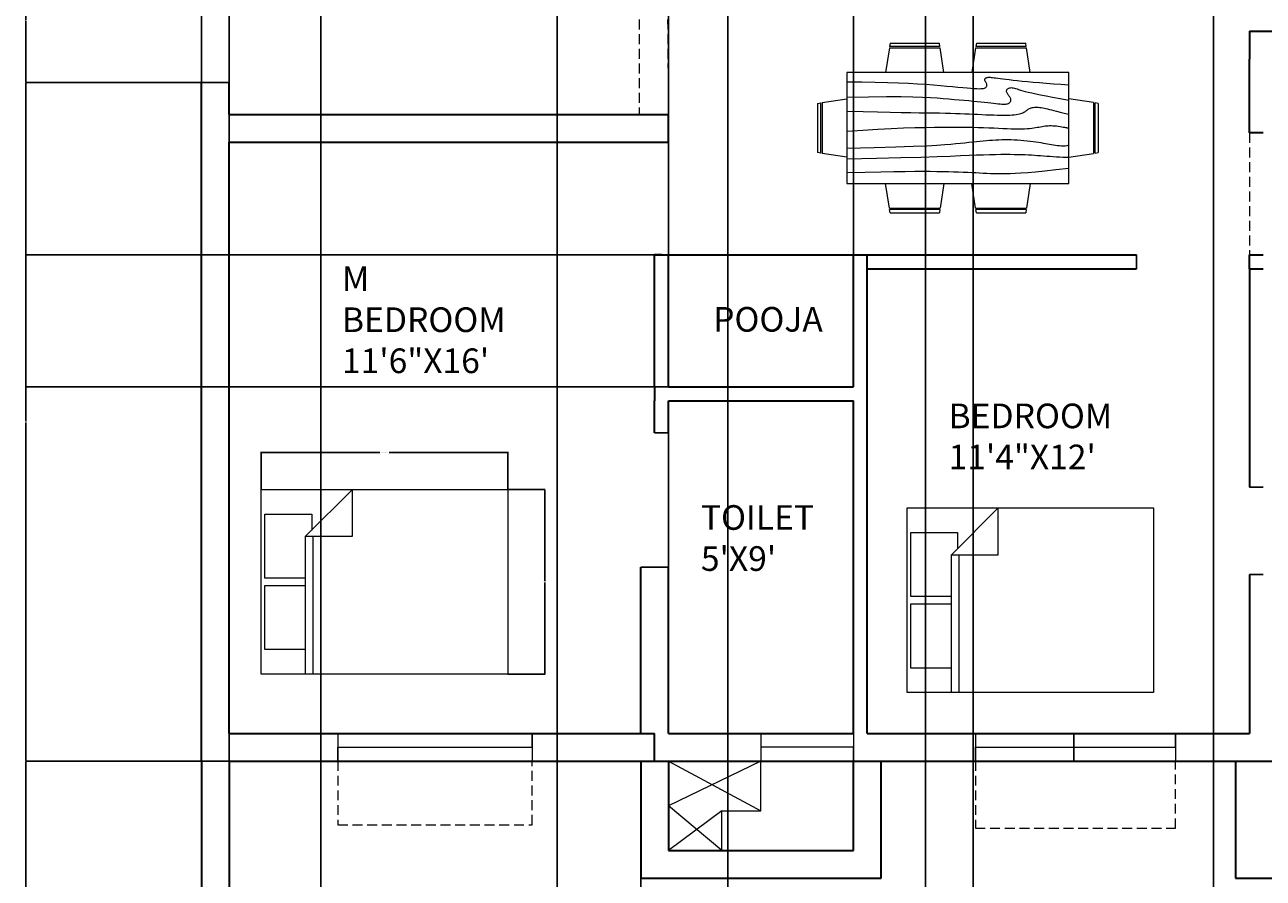
# Model space of a CAD drawing. Units: inches. Extents: x 276 to 912, y -567 to 621.
# Tile 5 of 7: x 276 to 678, y 65 to 342. Entities that reach past the tile are written whole.
import ezdxf

# ---------------------------------------------------------------- set-up
doc = ezdxf.new("R2010")
doc.units = ezdxf.units.IN
doc.linetypes.add('HIDDEN2', pattern=[4.7625, 3.175, -1.5875])
for name, color, linetype, lineweight in [('A-ANNO-DIMS', 2, 'Continuous', 18), ('A-AREA-IDEN', 7, 'Continuous', 18), ('A-DOOR', 3, 'Continuous', 25), ('A-FLOR-OVHD', 8, 'HIDDEN2', 13), ('A-FLOR-SHFT', 8, 'Continuous', 18), ('A-FURN', 8, 'Continuous', 18), ('A-GLAZ', 4, 'Continuous', 18), ('A-WALL', 7, 'Continuous', 35), ('A-WALL-HIDN', 8, 'HIDDEN2', 18)]:
    doc.layers.add(name, color=color, linetype=linetype, lineweight=lineweight)
doc.dimstyles.get("Standard").update_dxf_attribs({"dimtxt": 0.18, "dimasz": 0.18, "dimexe": 0.18, "dimexo": 0.0625, "dimgap": 0.09, "dimtad": 0, "dimtih": 1, "dimtoh": 1, "dimdec": 4, "dimzin": 0, "dimdsep": 46, "dimtxsty": 'Standard', "dimcen": 0.09, "dimadec": 0, "dimazin": 0, "dimtfac": 1, "dimtdec": 4, "dimtofl": 0, "dimtmove": 0, "dimatfit": 3, "dimfxl": 1, "dimtolj": 1, "dimtzin": 0, "dimarcsym": 0})

# ---------------------------------------------------------------- blocks, each defined once
blk = doc.blocks.new('Bed - Queen')
for p, q in [((0, -80.00003), (0, 0)), ((0, 0), (59.99999, 0)), ((59.99999, 0), (59.99999, -80.00003)), ((7.99999, -1.2), (28.79998, -1.2)), ((7.99999, -14.4), (7.99999, -1.2)), ((28.79998, -1.2), (28.79998, -14.4)), ((31.19999, -1.2), (51.99999, -1.2)), ((31.19999, -14.4), (31.19999, -1.2)), ((51.99999, -1.2), (51.99999, -16.4)), ((0, -14.4), (44.8, -14.4)), ((59.99999, -29.6), (44.8, -14.4)), ((44.8, -14.4), (44.8, -29.6)), ((44.8, -16.8), (0, -16.8)), ((51.99999, -16.4), (46.79936, -16.4)), ((44.8, -29.6), (59.99999, -29.6)), ((59.99999, -80.00003), (0, -80.00003))]:
    blk.add_line(p, q)
blk = doc.blocks.new('Dining Set - 36 x 72 in.')
for p, q in [((-22.2343, 26.00059), (-23.4847, 17.99762)), ((-22.2304, 26), (-5.7608, 26)), ((-22, 27.5), (-22.1562, 26.50042)), ((-5.8416, 26.5), (-22.1534, 26.5)), ((-22, 27.5), (-6, 27.5)), ((-5.8437, 26.49966), (-6, 27.5)), ((-4.5152, 17.99762), (-5.7655, 25.99926)), ((5.7657, 26.00059), (4.5153, 17.99762)), ((5.7696, 26), (22.2392, 26)), ((6, 27.5), (5.8438, 26.50042)), ((22.1584, 26.5), (5.8466, 26.5)), ((6, 27.5), (22, 27.5)), ((22.1563, 26.49966), (22, 27.5)), ((23.4848, 17.99762), (22.2345, 25.99926)), ((36, 18), (-36, 18)), ((-36, 18), (-36, -18)), ((36, -18), (36, 18)), ((-45.5, 8), (-44.5004, 8.15617)), ((-44.5, -8.15843), (-44.5, 8.15338)), ((-44.0006, 8.23428), (-35.9976, 9.48474)), ((-44, 8.23041), (-44, -8.23915)), ((44.0006, 8.23428), (35.9976, 9.48474)), ((44, 8.23041), (44, -8.23915)), ((44.5, -8.15843), (44.5, 8.15338)), ((45.5, 8), (44.5005, 8.15617)), ((-45.5, 8), (-45.5, -8)), ((45.5, 8), (45.5, -8)), ((-44.4997, -8.15631), (-45.5, -8)), ((44.4997, -8.15631), (45.5, -8)), ((-35.9976, -9.48476), (-43.9993, -8.2345)), ((35.9976, -9.48476), (43.9993, -8.2345)), ((-36, -18), (36, -18)), ((-22.2343, -26.0006), (-23.4847, -17.99762)), ((-4.5152, -17.99762), (-5.7655, -25.99928)), ((5.7657, -26.0006), (4.5153, -17.99762)), ((23.4848, -17.99762), (22.2345, -25.99928)), ((-22.2304, -26), (-5.7608, -26)), ((-22, -27.5), (-22.1562, -26.50044)), ((-5.8416, -26.5), (-22.1534, -26.5)), ((-22, -27.5), (-6, -27.5)), ((-5.8437, -26.49967), (-6, -27.5)), ((5.7696, -26), (22.2392, -26)), ((6, -27.5), (5.8438, -26.50044)), ((22.1584, -26.5), (5.8466, -26.5)), ((6, -27.5), (22, -27.5)), ((22.1563, -26.49967), (22, -27.5))]:
    blk.add_line(p, q)
for points in [[(-36, 15), (-31.1772, 14.97754), (-26.8079, 14.91406), (-22.8538, 14.81543), (-19.276, 14.6875), (-16.0362, 14.53613), (-13.0957, 14.36718), (-10.4159, 14.18652), (-7.9583, 14), (-5.6904, 13.81315), (-3.6035, 13.63021), (-1.6954, 13.45508), (0.0365, 13.29166), (1.5945, 13.14388), (2.9811, 13.01562), (4.1988, 12.9108), (5.25, 12.83333), (6.1393, 12.78613), (6.8802, 12.76823), (7.4883, 12.77767), (7.9792, 12.8125), (8.3685, 12.87077), (8.6719, 12.95052), (8.9049, 13.0498), (9.0833, 13.16666), (9.2205, 13.29899), (9.3216, 13.44401), (9.3895, 13.59879), (9.4271, 13.76041), (9.4373, 13.92594), (9.4232, 14.09245), (9.3875, 14.257), (9.3333, 14.41666), (9.2638, 14.56917), (9.1836, 14.71484), (9.0975, 14.85465), (9.0104, 14.98958), (8.9272, 15.1206), (8.8529, 15.2487), (8.7922, 15.37483), (8.75, 15.5), (8.7305, 15.62467), (8.7344, 15.74739), (8.7617, 15.86621), (8.8125, 15.97916), (8.8867, 16.08431), (8.9844, 16.17968), (9.1055, 16.26334), (9.25, 16.33333), (9.4189, 16.38802), (9.6172, 16.42708), (9.8506, 16.45052), (10.125, 16.45833), (10.4463, 16.45052), (10.8203, 16.42708), (11.2529, 16.38802), (11.75, 16.33333), (12.3184, 16.26318), (12.9694, 16.17838), (13.7151, 16.07991), (14.5677, 15.96875), (15.5395, 15.84586), (16.6426, 15.71224), (17.8893, 15.56884), (19.2917, 15.41666), (20.859, 15.25667), (22.5879, 15.08984), (24.4721, 14.91715), (26.5052, 14.73958), (28.6809, 14.5581), (30.9929, 14.3737), (33.4347, 14.18733), (36, 14)], [(-36, 10), (-28.9766, 10.14274), (-23.1725, 10.20442), (-18.4241, 10.19775), (-14.5677, 10.13541), (-11.4399, 10.03011), (-8.877, 9.89453), (-6.7154, 9.74137), (-4.7917, 9.58333), (-2.9698, 9.43082), (-1.2246, 9.28515), (0.4415, 9.14534), (2.026, 9.01041), (3.5266, 8.87939), (4.9408, 8.7513), (6.266, 8.62516), (7.5, 8.5), (8.6411, 8.37549), (9.6914, 8.2539), (10.6538, 8.13818), (11.5312, 8.03125), (12.3267, 7.93603), (13.043, 7.85547), (13.6831, 7.79248), (14.25, 7.75), (14.7471, 7.7303), (15.1797, 7.73307), (15.5537, 7.75732), (15.875, 7.80208), (16.1494, 7.86637), (16.3828, 7.94922), (16.5811, 8.04964), (16.75, 8.16666), (16.8944, 8.29915), (17.0143, 8.44531), (17.1089, 8.60319), (17.1771, 8.77083), (17.218, 8.94629), (17.2305, 9.1276), (17.2137, 9.31282), (17.1667, 9.5), (17.0895, 9.6875), (16.987, 9.875), (16.8649, 10.0625), (16.7292, 10.25), (16.5856, 10.4375), (16.4401, 10.625), (16.2985, 10.8125), (16.1667, 11), (16.05, 11.18733), (15.9518, 11.3737), (15.8752, 11.5581), (15.8229, 11.73958), (15.798, 11.91715), (15.8034, 12.08984), (15.842, 12.25667), (15.9167, 12.41666), (16.0295, 12.56836), (16.1784, 12.70833), (16.3605, 12.83268), (16.5729, 12.9375), (16.8127, 13.01888), (17.0768, 13.07291), (17.3625, 13.0957), (17.6667, 13.08333), (17.9894, 13.03312), (18.3418, 12.94726), (18.7382, 12.82918), (19.1927, 12.68229), (19.7195, 12.51001), (20.3327, 12.31575), (21.0465, 12.10294), (21.875, 11.875), (22.8357, 11.63354), (23.959, 11.37304), (25.2786, 11.08618), (26.8282, 10.76562), (28.6414, 10.40405), (30.752, 9.99414), (33.1936, 9.52856), (36, 9)], [(-36, 5.5), (-30.7157, 5.3348), (-26.069, 5.20963), (-21.9946, 5.11767), (-18.4271, 5.05208), (-15.3009, 5.00602), (-12.5508, 4.97265), (-10.1112, 4.94515), (-7.9167, 4.91666), (-5.909, 4.88167), (-4.0586, 4.83984), (-2.3429, 4.79215), (-0.7396, 4.73958), (0.7739, 4.6831), (2.22, 4.6237), (3.6213, 4.56233), (5, 4.5), (6.373, 4.43782), (7.7344, 4.3776), (9.0723, 4.32129), (10.375, 4.27083), (11.6309, 4.22819), (12.8281, 4.19531), (13.9551, 4.17415), (15, 4.16666), (15.954, 4.17448), (16.819, 4.19791), (17.6001, 4.23698), (18.3021, 4.29166), (18.9299, 4.36198), (19.4883, 4.44791), (19.9823, 4.54948), (20.4167, 4.66666), (20.7969, 4.79899), (21.1302, 4.94401), (21.4245, 5.09879), (21.6875, 5.26041), (21.9271, 5.42594), (22.1511, 5.59245), (22.3672, 5.757), (22.5834, 5.91666), (22.8065, 6.06868), (23.0404, 6.21093), (23.2879, 6.34147), (23.5521, 6.45833), (23.8358, 6.55957), (24.142, 6.64323), (24.4735, 6.70735), (24.8334, 6.75), (25.2235, 6.76969), (25.642, 6.76692), (26.0858, 6.74267), (26.5521, 6.69791), (27.0379, 6.63362), (27.5404, 6.55078), (28.0565, 6.45036), (28.5834, 6.33333), (29.1242, 6.19987), (29.7071, 6.04687), (30.3661, 5.87044), (31.1354, 5.66666), (32.0493, 5.43164), (33.142, 5.16146), (34.4475, 4.85221), (36, 4.5)], [(-36, -1), (-30.7915, -0.6591), (-26.0195, -0.38216), (-21.6519, -0.16284), (-17.6563, 0.00521), (-14.0005, 0.12833), (-10.6523, 0.21289), (-7.5796, 0.26522), (-4.75, 0.29166), (-2.134, 0.29793), (0.2878, 0.28711), (2.5317, 0.26163), (4.6146, 0.22396), (6.5529, 0.17651), (8.3633, 0.12174), (10.0623, 0.06209), (11.6667, 0), (13.1899, -0.06201), (14.6341, -0.1211), (15.9982, -0.17432), (17.2813, -0.21875), (18.4823, -0.25147), (19.6003, -0.26953), (20.6343, -0.27002), (21.5834, -0.25), (22.4481, -0.20768), (23.2357, -0.14584), (23.9549, -0.06836), (24.6146, 0.02083), (25.2235, 0.11784), (25.7904, 0.21875), (26.3241, 0.31966), (26.8334, 0.41666), (27.3265, 0.50618), (27.8099, 0.58593), (28.2894, 0.65397), (28.7709, 0.70833), (29.2601, 0.74707), (29.763, 0.76823), (30.2855, 0.76985), (30.8334, 0.75), (31.4088, 0.70784), (31.9994, 0.64713), (32.589, 0.57275), (33.1615, 0.48958), (33.7008, 0.4025), (34.1908, 0.3164), (34.6153, 0.23616), (34.9584, 0.16666), (35.2099, 0.11165), (35.3848, 0.07031), (35.504, 0.04069), (35.5886, 0.02083), (35.6594, 0.00879), (35.7377, 0.0026), (35.8442, 0.00032), (36, 0)], [(-36, -6.5), (-27.1843, -6.31267), (-20.084, -6.1263), (-14.469, -5.9419), (-10.1094, -5.76042), (-6.7752, -5.58285), (-4.2363, -5.41016), (-2.2629, -5.24333), (-0.625, -5.08334), (0.8708, -4.93099), (2.2715, -4.78646), (3.5872, -4.64974), (4.8281, -4.52084), (6.0046, -4.39974), (7.127, -4.28646), (8.2053, -4.18099), (9.25, -4.08334), (10.2705, -3.99382), (11.2734, -3.91407), (12.2647, -3.84603), (13.25, -3.79167), (14.2354, -3.75293), (15.2266, -3.73177), (16.2295, -3.73015), (17.25, -3.75), (18.2912, -3.79248), (19.3451, -3.85547), (20.4009, -3.93604), (21.4479, -4.03125), (22.4754, -4.13819), (23.4727, -4.25391), (24.4289, -4.37549), (25.3334, -4.5), (26.1785, -4.62492), (26.9694, -4.74935), (27.7145, -4.87281), (28.4219, -4.99479), (29.1, -5.11483), (29.7572, -5.23242), (30.4016, -5.34709), (31.0417, -5.45834), (31.6837, -5.56437), (32.3262, -5.65821), (32.9658, -5.73153), (33.599, -5.77604), (34.2224, -5.78345), (34.8327, -5.74545), (35.4264, -5.65373), (36, -5.5)], [(-36, -10), (-26.4022, -9.81299), (-18.4675, -9.62891), (-11.9839, -9.45069), (-6.7396, -9.28125), (-2.5226, -9.12354), (0.8789, -8.98047), (3.6769, -8.85498), (6.0833, -8.75), (8.2767, -8.66765), (10.3021, -8.60677), (12.1712, -8.56543), (13.8958, -8.54167), (15.4876, -8.53353), (16.9583, -8.53907), (18.3197, -8.55632), (19.5834, -8.58334), (20.7616, -8.61841), (21.8685, -8.66081), (22.9188, -8.71004), (23.9271, -8.76563), (24.9081, -8.82707), (25.8763, -8.89388), (26.8465, -8.96558), (27.8334, -9.04167), (28.8474, -9.12118), (29.8828, -9.20117), (30.93, -9.27824), (31.9792, -9.34896), (33.0205, -9.40991), (34.0443, -9.45768), (35.0407, -9.48885), (36, -9.5)], [(-36, -14.5), (-30.0881, -14.33513), (-25.0332, -14.21224), (-20.7312, -14.12647), (-17.0781, -14.07292), (-13.97, -14.04671), (-11.3027, -14.04297), (-8.9724, -14.05681), (-6.875, -14.08334), (-4.9224, -14.11833), (-3.0905, -14.16016), (-1.3709, -14.20785), (0.2448, -14.26042), (1.7647, -14.3169), (3.1973, -14.3763), (4.5507, -14.43767), (5.8333, -14.5), (7.0554, -14.5621), (8.235, -14.62175), (9.3922, -14.67652), (10.5469, -14.72396), (11.7192, -14.76164), (12.929, -14.78711), (14.1965, -14.79794), (15.5417, -14.79167), (16.9933, -14.76424), (18.6152, -14.70508), (20.4804, -14.60197), (22.6615, -14.44271), (25.2312, -14.21509), (28.2624, -13.9069), (31.8277, -13.50594), (36, -13)]]:
    blk.add_lwpolyline(points)
blk = doc.blocks.new('DOOR-JAMB-4.5IN')
for p, q in [((0, 2.25), (0, 4.5)), ((0, 4.5), (0, 0))]:
    blk.add_line(p, q)
blk = doc.blocks.new('*D12')
at = {"layer": 'A-ANNO-DIMS', "color": 0, "lineweight": -2, "transparency": 16777216}
for p, q in [((352.43, 191.61), (352.43, 203.73)), ((352.61, 203.55), (390.91, 203.55)), ((432.25, 203.55), (393.94, 203.55)), ((432.43, 191.61), (432.43, 203.73))]:
    blk.add_line(p, q, dxfattribs=at)
at = {"layer": 'A-ANNO-DIMS', "color": 0, "transparency": 16777216}
for points in [[(352.61, 203.58), (352.61, 203.52), (352.43, 203.55)], [(432.25, 203.58), (432.25, 203.52), (432.43, 203.55)]]:
    blk.add_solid(points, dxfattribs=at)
at = {"layer": 'Defpoints', "color": 0, "transparency": 16777216}
for p in [(352.43, 203.55), (352.43, 191.55), (432.43, 191.55)]:
    blk.add_point(p, dxfattribs=at)
at = {"layer": 'A-ANNO-DIMS', "color": 0, "transparency": 16777216, "insert": (392.43, 203.55), "char_height": 0.18, "attachment_point": 5}
blk.add_mtext('\\A1;QUEEN BED 80 TYP.', dxfattribs=at)
blk = doc.blocks.new('*D13')
at = {"layer": 'A-ANNO-DIMS', "color": 0, "lineweight": -2, "transparency": 16777216}
for p, q in [((432.49, 191.55), (444.61, 191.55)), ((444.43, 191.37), (444.43, 161.73)), ((444.43, 131.73), (444.43, 161.37)), ((432.49, 131.55), (444.61, 131.55))]:
    blk.add_line(p, q, dxfattribs=at)
at = {"layer": 'A-ANNO-DIMS', "color": 0, "transparency": 16777216}
for points in [[(444.4, 191.37), (444.46, 191.37), (444.43, 191.55)], [(444.4, 131.73), (444.46, 131.73), (444.43, 131.55)]]:
    blk.add_solid(points, dxfattribs=at)
at = {"layer": 'Defpoints', "color": 0, "transparency": 16777216}
for p in [(432.43, 191.55), (444.43, 191.55), (432.43, 131.55)]:
    blk.add_point(p, dxfattribs=at)
at = {"layer": 'A-ANNO-DIMS', "color": 0, "transparency": 16777216, "insert": (444.43, 161.55), "char_height": 0.18, "attachment_point": 5}
blk.add_mtext('\\A1;60 TYP.', dxfattribs=at)
blk = doc.blocks.new('*D24')
at = {"layer": 'A-ANNO-DIMS', "color": 0, "lineweight": -2, "transparency": 16777216}
for p, q in [((333.082179, 103.255751), (333.082179, -553.223061)), ((854.209085, -327.604004), (854.209085, -553.223061)), ((333.262179, -553.043061), (593.255632, -553.043061)), ((854.029085, -553.043061), (594.035632, -553.043061))]:
    blk.add_line(p, q, dxfattribs=at)
at = {"layer": 'A-ANNO-DIMS', "color": 0, "transparency": 16777216}
for points in [[(333.262179, -553.013061), (333.262179, -553.073061), (333.082179, -553.043061)], [(854.029085, -553.013061), (854.029085, -553.073061), (854.209085, -553.043061)]]:
    blk.add_solid(points, dxfattribs=at)
at = {"layer": 'Defpoints', "color": 0, "transparency": 16777216}
for p in [(333.082179, 103.318251), (854.209085, -327.541504), (854.209085, -553.043061)]:
    blk.add_point(p, dxfattribs=at)
at = {"layer": 'A-ANNO-DIMS', "color": 0, "transparency": 16777216, "insert": (593.645632, -553.043061), "char_height": 0.18, "attachment_point": 5}
blk.add_mtext('\\A1;521.1', dxfattribs=at)
blk = doc.blocks.new('*D25')
at = {"layer": 'A-ANNO-DIMS', "color": 0, "lineweight": -2, "transparency": 16777216}
for p, q in [((478.5, 564.29), (911.39, 564.29)), ((911.21, 564.11), (911.21, 34.31)), ((911.21, -495.86), (911.21, 33.95)), ((582.98, -496.04), (911.39, -496.04))]:
    blk.add_line(p, q, dxfattribs=at)
at = {"layer": 'A-ANNO-DIMS', "color": 0, "transparency": 16777216}
for points in [[(911.18, 564.11), (911.24, 564.11), (911.21, 564.29)], [(911.18, -495.86), (911.24, -495.86), (911.21, -496.04)]]:
    blk.add_solid(points, dxfattribs=at)
at = {"layer": 'Defpoints', "color": 0, "transparency": 16777216}
for p in [(478.44, 564.29), (582.92, -496.04), (911.21, -496.04)]:
    blk.add_point(p, dxfattribs=at)
at = {"layer": 'A-ANNO-DIMS', "color": 0, "transparency": 16777216, "insert": (911.21, 34.13), "char_height": 0.18, "attachment_point": 5}
blk.add_mtext('\\A1;1060.3', dxfattribs=at)
blk = doc.blocks.new('*D26')
at = {"layer": 'A-ANNO-DIMS', "color": 0, "lineweight": -2, "transparency": 16777216}
for p, q in [((342.02, 103.32), (275.9, 103.32)), ((276.08, 103.14), (276.08, 19.57)), ((276.08, -64.36), (276.08, 19.21)), ((342.02, -64.54), (275.9, -64.54))]:
    blk.add_line(p, q, dxfattribs=at)
at = {"layer": 'A-ANNO-DIMS', "color": 0, "transparency": 16777216}
for points in [[(276.05, 103.14), (276.11, 103.14), (276.08, 103.32)], [(276.05, -64.36), (276.11, -64.36), (276.08, -64.54)]]:
    blk.add_solid(points, dxfattribs=at)
at = {"layer": 'Defpoints', "color": 0, "transparency": 16777216}
for p in [(342.08, 103.32), (276.08, -64.54), (342.08, -64.54)]:
    blk.add_point(p, dxfattribs=at)
at = {"layer": 'A-ANNO-DIMS', "color": 0, "transparency": 16777216, "insert": (276.08, 19.39), "char_height": 0.18, "attachment_point": 5}
blk.add_mtext('\\A1;167.86', dxfattribs=at)
blk = doc.blocks.new('*D31')
at = {"layer": 'A-ANNO-DIMS', "color": 0, "lineweight": -2, "transparency": 16777216}
for p, q in [((333.082179, 103.255751), (333.082179, -553.223061)), ((475.582179, 65.246155), (475.582179, -553.223061)), ((333.262179, -553.043061), (403.912179, -553.043061)), ((475.402179, -553.043061), (404.752179, -553.043061))]:
    blk.add_line(p, q, dxfattribs=at)
at = {"layer": 'A-ANNO-DIMS', "color": 0, "transparency": 16777216}
for points in [[(333.262179, -553.013061), (333.262179, -553.073061), (333.082179, -553.043061)], [(475.402179, -553.013061), (475.402179, -553.073061), (475.582179, -553.043061)]]:
    blk.add_solid(points, dxfattribs=at)
at = {"layer": 'Defpoints', "color": 0, "transparency": 16777216}
for p in [(333.082179, 103.318251), (475.582179, 65.308655), (475.582179, -553.043061)]:
    blk.add_point(p, dxfattribs=at)
at = {"layer": 'A-ANNO-DIMS', "color": 0, "transparency": 16777216, "insert": (404.332179, -553.043061), "char_height": 0.18, "attachment_point": 5}
blk.add_mtext('\\A1;142.5', dxfattribs=at)
blk = doc.blocks.new('*D37')
at = {"layer": 'A-ANNO-DIMS', "color": 0, "lineweight": -2, "transparency": 16777216}
for p, q in [((333.019679, 363.831643), (275.902179, 363.831643)), ((276.082179, 363.651643), (276.082179, 343.929428)), ((276.082179, 323.847213), (276.082179, 343.569428)), ((333.019679, 323.667213), (275.902179, 323.667213))]:
    blk.add_line(p, q, dxfattribs=at)
at = {"layer": 'A-ANNO-DIMS', "color": 0, "transparency": 16777216}
for points in [[(276.052179, 363.651643), (276.112179, 363.651643), (276.082179, 363.831643)], [(276.052179, 323.847213), (276.112179, 323.847213), (276.082179, 323.667213)]]:
    blk.add_solid(points, dxfattribs=at)
at = {"layer": 'Defpoints', "color": 0, "transparency": 16777216}
for p in [(276.082179, 363.831643), (333.082179, 363.831643), (333.082179, 323.667213)]:
    blk.add_point(p, dxfattribs=at)
at = {"layer": 'A-ANNO-DIMS', "color": 0, "transparency": 16777216, "insert": (276.082179, 343.749428), "char_height": 0.18, "attachment_point": 5}
blk.add_mtext('\\A1;40.164', dxfattribs=at)
blk = doc.blocks.new('*D38')
at = {"layer": 'A-ANNO-DIMS', "color": 0, "lineweight": -2, "transparency": 16777216}
for p, q in [((333.019679, 323.667213), (275.902179, 323.667213)), ((276.082179, 323.487213), (276.082179, 213.672732)), ((276.082179, 103.498251), (276.082179, 213.312732)), ((333.019679, 103.318251), (275.902179, 103.318251))]:
    blk.add_line(p, q, dxfattribs=at)
at = {"layer": 'A-ANNO-DIMS', "color": 0, "transparency": 16777216}
for points in [[(276.052179, 323.487213), (276.112179, 323.487213), (276.082179, 323.667213)], [(276.052179, 103.498251), (276.112179, 103.498251), (276.082179, 103.318251)]]:
    blk.add_solid(points, dxfattribs=at)
at = {"layer": 'Defpoints', "color": 0, "transparency": 16777216}
for p in [(276.082179, 323.667213), (333.082179, 323.667213), (333.082179, 103.318251)]:
    blk.add_point(p, dxfattribs=at)
at = {"layer": 'A-ANNO-DIMS', "color": 0, "transparency": 16777216, "insert": (276.082179, 213.492732), "char_height": 0.18, "attachment_point": 5}
blk.add_mtext('\\A1;220.35', dxfattribs=at)
blk = doc.blocks.new('*D41')
at = {"layer": 'A-ANNO-DIMS', "color": 0, "lineweight": -2, "transparency": 16777216}
for p, q in [((333.082179, 363.769143), (333.082179, -553.223061)), ((342.082179, 363.769143), (342.082179, -553.223061)), ((333.262179, -553.043061), (337.432179, -553.043061)), ((341.902179, -553.043061), (337.732179, -553.043061))]:
    blk.add_line(p, q, dxfattribs=at)
at = {"layer": 'A-ANNO-DIMS', "color": 0, "transparency": 16777216}
for points in [[(333.262179, -553.013061), (333.262179, -553.073061), (333.082179, -553.043061)], [(341.902179, -553.013061), (341.902179, -553.073061), (342.082179, -553.043061)]]:
    blk.add_solid(points, dxfattribs=at)
at = {"layer": 'Defpoints', "color": 0, "transparency": 16777216}
for p in [(333.082179, 363.831643), (342.082179, 363.831643), (342.082179, -553.043061)]:
    blk.add_point(p, dxfattribs=at)
at = {"layer": 'A-ANNO-DIMS', "color": 0, "transparency": 16777216, "insert": (337.582179, -553.043061), "char_height": 0.18, "attachment_point": 5}
blk.add_mtext('\\A1;9', dxfattribs=at)
blk = doc.blocks.new('*D42')
at = {"layer": 'A-ANNO-DIMS', "color": 0, "lineweight": -2, "transparency": 16777216}
for p, q in [((484.582179, 267.783946), (484.582179, 621.473746)), ((484.762179, 621.293746), (514.357179, 621.293746)), ((544.402179, 621.293746), (514.807179, 621.293746)), ((544.582179, 267.783946), (544.582179, 621.473746))]:
    blk.add_line(p, q, dxfattribs=at)
at = {"layer": 'A-ANNO-DIMS', "color": 0, "transparency": 16777216}
for points in [[(484.762179, 621.323746), (484.762179, 621.263746), (484.582179, 621.293746)], [(544.402179, 621.323746), (544.402179, 621.263746), (544.582179, 621.293746)]]:
    blk.add_solid(points, dxfattribs=at)
at = {"layer": 'Defpoints', "color": 0, "transparency": 16777216}
for p in [(544.582179, 621.293746), (484.582179, 267.721446), (544.582179, 267.721446)]:
    blk.add_point(p, dxfattribs=at)
at = {"layer": 'A-ANNO-DIMS', "color": 0, "transparency": 16777216, "insert": (514.582179, 621.293746), "char_height": 0.18, "attachment_point": 5}
blk.add_mtext('\\A1;60', dxfattribs=at)
blk = doc.blocks.new('*D43')
at = {"layer": 'A-ANNO-DIMS', "color": 0, "lineweight": -2, "transparency": 16777216}
for p, q in [((484.52, 267.72), (275.9, 267.72)), ((276.08, 267.54), (276.08, 246.45)), ((276.08, 225), (276.08, 246.09)), ((484.52, 224.82), (275.9, 224.82))]:
    blk.add_line(p, q, dxfattribs=at)
at = {"layer": 'A-ANNO-DIMS', "color": 0, "transparency": 16777216}
for points in [[(276.05, 267.54), (276.11, 267.54), (276.08, 267.72)], [(276.05, 225), (276.11, 225), (276.08, 224.82)]]:
    blk.add_solid(points, dxfattribs=at)
at = {"layer": 'Defpoints', "color": 0, "transparency": 16777216}
for p in [(276.08, 267.72), (484.58, 267.72), (484.58, 224.82)]:
    blk.add_point(p, dxfattribs=at)
at = {"layer": 'A-ANNO-DIMS', "color": 0, "transparency": 16777216, "insert": (276.08, 246.27), "char_height": 0.18, "attachment_point": 5}
blk.add_mtext('\\A1;42.9', dxfattribs=at)
blk = doc.blocks.new('*D59')
at = {"layer": 'A-ANNO-DIMS', "color": 0, "lineweight": -2, "transparency": 16777216}
for p, q in [((333.082179, -81.315568), (333.082179, 621.473746)), ((333.262179, 621.293746), (457.725334, 621.293746)), ((583.238489, 621.293746), (458.775334, 621.293746)), ((583.418489, -30.671128), (583.418489, 621.473746))]:
    blk.add_line(p, q, dxfattribs=at)
at = {"layer": 'A-ANNO-DIMS', "color": 0, "transparency": 16777216}
for points in [[(333.262179, 621.323746), (333.262179, 621.263746), (333.082179, 621.293746)], [(583.238489, 621.323746), (583.238489, 621.263746), (583.418489, 621.293746)]]:
    blk.add_solid(points, dxfattribs=at)
at = {"layer": 'Defpoints', "color": 0, "transparency": 16777216}
for p in [(583.418489, 621.293746), (583.418489, -30.733628), (333.082179, -81.378068)]:
    blk.add_point(p, dxfattribs=at)
at = {"layer": 'A-ANNO-DIMS', "color": 0, "transparency": 16777216, "insert": (458.250334, 621.293746), "char_height": 0.18, "attachment_point": 5}
blk.add_mtext('\\A1;250.34', dxfattribs=at)
blk = doc.blocks.new('*D60')
at = {"layer": 'A-ANNO-DIMS', "color": 0, "lineweight": -2, "transparency": 16777216}
for p, q in [((583.418489, -30.671128), (583.418489, 621.473746)), ((583.598489, 621.293746), (622.178489, 621.293746)), ((661.238489, 621.293746), (622.658489, 621.293746)), ((661.418489, -30.671128), (661.418489, 621.473746))]:
    blk.add_line(p, q, dxfattribs=at)
at = {"layer": 'A-ANNO-DIMS', "color": 0, "transparency": 16777216}
for points in [[(583.598489, 621.323746), (583.598489, 621.263746), (583.418489, 621.293746)], [(661.238489, 621.323746), (661.238489, 621.263746), (661.418489, 621.293746)]]:
    blk.add_solid(points, dxfattribs=at)
at = {"layer": 'Defpoints', "color": 0, "transparency": 16777216}
for p in [(661.418489, 621.293746), (583.418489, -30.733628), (661.418489, -30.733628)]:
    blk.add_point(p, dxfattribs=at)
at = {"layer": 'A-ANNO-DIMS', "color": 0, "transparency": 16777216, "insert": (622.418489, 621.293746), "char_height": 0.18, "attachment_point": 5}
blk.add_mtext('\\A1;78', dxfattribs=at)
blk = doc.blocks.new('*D61')
at = {"layer": 'A-ANNO-DIMS', "color": 0, "lineweight": -2, "transparency": 16777216}
for p, q in [((661.418489, -30.671128), (661.418489, 621.473746)), ((661.598489, 621.293746), (741.263489, 621.293746)), ((821.738489, 621.293746), (742.073489, 621.293746)), ((821.918489, -64.479004), (821.918489, 621.473746))]:
    blk.add_line(p, q, dxfattribs=at)
at = {"layer": 'A-ANNO-DIMS', "color": 0, "transparency": 16777216}
for points in [[(661.598489, 621.323746), (661.598489, 621.263746), (661.418489, 621.293746)], [(821.738489, 621.323746), (821.738489, 621.263746), (821.918489, 621.293746)]]:
    blk.add_solid(points, dxfattribs=at)
at = {"layer": 'Defpoints', "color": 0, "transparency": 16777216}
for p in [(821.918489, 621.293746), (661.418489, -30.733628), (821.918489, -64.541504)]:
    blk.add_point(p, dxfattribs=at)
at = {"layer": 'A-ANNO-DIMS', "color": 0, "transparency": 16777216, "insert": (741.668489, 621.293746), "char_height": 0.18, "attachment_point": 5}
blk.add_mtext('\\A1;160.5', dxfattribs=at)
blk = doc.blocks.new('*D65')
at = {"layer": 'A-ANNO-DIMS', "color": 0, "lineweight": -2, "transparency": 16777216}
for p, q in [((342.08, -229.93), (342.08, 621.47)), ((342.26, 621.29), (356.48, 621.29)), ((371.59, 621.29), (357.38, 621.29)), ((371.77, -229.93), (371.77, 621.47))]:
    blk.add_line(p, q, dxfattribs=at)
at = {"layer": 'A-ANNO-DIMS', "color": 0, "transparency": 16777216}
for points in [[(342.26, 621.32), (342.26, 621.26), (342.08, 621.29)], [(371.59, 621.32), (371.59, 621.26), (371.77, 621.29)]]:
    blk.add_solid(points, dxfattribs=at)
at = {"layer": 'Defpoints', "color": 0, "transparency": 16777216}
for p in [(371.77, 621.29), (342.08, -229.99), (371.77, -229.99)]:
    blk.add_point(p, dxfattribs=at)
at = {"layer": 'A-ANNO-DIMS', "color": 0, "transparency": 16777216, "insert": (356.93, 621.29), "char_height": 0.18, "attachment_point": 5}
blk.add_mtext('\\A1;29.69', dxfattribs=at)
blk = doc.blocks.new('*D70')
at = {"layer": 'A-ANNO-DIMS', "color": 0, "lineweight": -2, "transparency": 16777216}
for p, q in [((448.42, -73.48), (448.42, 621.47)), ((448.6, 621.29), (475.69, 621.29)), ((503.69, 621.29), (476.59, 621.29)), ((503.87, -45.06), (503.87, 621.47))]:
    blk.add_line(p, q, dxfattribs=at)
at = {"layer": 'A-ANNO-DIMS', "color": 0, "transparency": 16777216}
for points in [[(448.6, 621.32), (448.6, 621.26), (448.42, 621.29)], [(503.69, 621.32), (503.69, 621.26), (503.87, 621.29)]]:
    blk.add_solid(points, dxfattribs=at)
at = {"layer": 'Defpoints', "color": 0, "transparency": 16777216}
for p in [(503.87, 621.29), (503.87, -45.12), (448.42, -73.54)]:
    blk.add_point(p, dxfattribs=at)
at = {"layer": 'A-ANNO-DIMS', "color": 0, "transparency": 16777216, "insert": (476.14, 621.29), "char_height": 0.18, "attachment_point": 5}
blk.add_mtext('\\A1;55.45', dxfattribs=at)
blk = doc.blocks.new('*D71')
at = {"layer": 'A-ANNO-DIMS', "color": 0, "lineweight": -2, "transparency": 16777216}
for p, q in [((503.866476, -45.059003), (503.866476, 621.473746)), ((504.046476, 621.293746), (535.522963, 621.293746)), ((567.83945, 621.293746), (536.362963, 621.293746)), ((568.01945, -45.059003), (568.01945, 621.473746))]:
    blk.add_line(p, q, dxfattribs=at)
at = {"layer": 'A-ANNO-DIMS', "color": 0, "transparency": 16777216}
for points in [[(504.046476, 621.323746), (504.046476, 621.263746), (503.866476, 621.293746)], [(567.83945, 621.323746), (567.83945, 621.263746), (568.01945, 621.293746)]]:
    blk.add_solid(points, dxfattribs=at)
at = {"layer": 'Defpoints', "color": 0, "transparency": 16777216}
for p in [(568.01945, 621.293746), (503.866476, -45.121503), (568.01945, -45.121503)]:
    blk.add_point(p, dxfattribs=at)
at = {"layer": 'A-ANNO-DIMS', "color": 0, "transparency": 16777216, "insert": (535.942963, 621.293746), "char_height": 0.18, "attachment_point": 5}
blk.add_mtext('\\A1;64.15', dxfattribs=at)

msp = doc.modelspace()

# ---------------------------------------------------------------- linework, layer by layer
at = {"layer": 'A-DOOR'}
for p, q in [((333.0822, 323.6672), (342.0822, 323.6672)), ((480.0822, 209.9053), (484.5822, 209.9053)), ((484.5822, 166.3183), (484.5822, 209.9053)), ((475.5822, 166.3183), (484.5822, 166.3183))]:
    msp.add_line(p, q, dxfattribs=at)
at = {"layer": 'A-FLOR-OVHD'}
for p, q in [((377.3113, 103.3183), (377.3113, 82.6995)), ((440.3707, 82.6995), (440.3707, 103.3183)), ((584.2252, 103.3183), (584.2252, 81.5744)), ((649.1043, 81.5744), (649.1043, 103.3183)), ((377.3113, 82.6995), (440.3707, 82.6995)), ((584.2252, 81.5744), (649.1043, 81.5744))]:
    msp.add_line(p, q, dxfattribs=at)
at = {"layer": 'A-FLOR-SHFT'}
for p, q in [((514.5822, 103.3183), (484.5822, 88.8135)), ((484.5822, 103.3183), (514.5822, 87.1973)), ((514.5822, 87.1973), (514.5822, 103.3183)), ((501.9024, 74.3087), (484.5822, 88.8135)), ((501.9024, 87.1973), (484.5822, 74.3087)), ((501.9024, 74.3087), (501.9024, 87.1973)), ((501.9024, 87.1973), (514.5822, 87.1973))]:
    msp.add_line(p, q, dxfattribs=at)
at = {"layer": 'A-GLAZ'}
for p, q in [((377.3113, 112.3183), (377.3113, 103.3183)), ((440.3707, 107.8183), (440.3707, 112.3183)), ((440.3707, 112.3183), (440.3707, 103.3183)), ((514.5822, 112.3183), (514.5822, 103.3183)), ((544.5822, 112.3183), (544.5822, 103.3183)), ((377.3113, 103.3183), (377.3113, 107.8183)), ((377.3113, 107.8183), (440.3707, 107.8183)), ((544.5822, 107.8183), (514.5822, 107.8183)), ((544.5822, 103.3183), (544.5822, 107.8183))]:
    msp.add_line(p, q, dxfattribs=at)
msp.add_lwpolyline([(584.2252, 112.3183), (584.2252, 112.3183), (584.2252, 103.3183), (584.2252, 107.8183), (616.1716, 107.8183), (616.1716, 112.3183), (616.1716, 103.3183), (616.1716, 107.8183), (649.1043, 107.8183), (649.1043, 112.3183), (649.1043, 103.3183)], dxfattribs=at)
at = {"layer": 'A-WALL'}
for p, q in [((673.0822, 340.3183), (673.0822, 331.3183)), ((673.0822, 340.3183), (818.5822, 340.3183)), ((673.0822, 307.3183), (673.0822, 331.3183)), ((333.0822, 103.3183), (333.0822, 323.6672)), ((342.0822, 313.3183), (342.0822, 323.6672)), ((342.0822, 313.3183), (484.0822, 313.3183)), ((484.0822, 313.3183), (484.5822, 313.3183)), ((484.5822, 304.3183), (484.5822, 313.3183)), ((677.5822, 307.3183), (673.0822, 307.3183)), ((342.0822, 304.3183), (484.0822, 304.3183)), ((342.0822, 224.8183), (342.0822, 304.3183)), ((484.0822, 304.3183), (484.5822, 304.3183)), ((482.3898, 267.7214), (480.0822, 267.7214)), ((480.0822, 267.7214), (484.5822, 267.7214)), ((480.0822, 224.8183), (480.0822, 267.7214)), ((484.5822, 267.7214), (549.0822, 267.7214)), ((484.5822, 224.8183), (484.5822, 267.7214)), ((544.5822, 224.8183), (544.5822, 267.7214)), ((549.0822, 112.3183), (549.0822, 267.7214)), ((549.0822, 267.7214), (636.4818, 267.7214)), ((673.0822, 263.2214), (673.0822, 267.7214)), ((673.0822, 267.7214), (677.5822, 267.7214)), ((549.0822, 263.2214), (636.4818, 263.2214)), ((673.0822, 263.2214), (673.0822, 192.2677)), ((673.0822, 263.2214), (677.5822, 263.2214)), ((342.0822, 220.3183), (342.0822, 224.8183)), ((480.0822, 224.8183), (480.0822, 220.3183)), ((484.5822, 224.8183), (544.5822, 224.8183)), ((484.5822, 224.8183), (544.5822, 224.8183)), ((342.0822, 112.3183), (342.0822, 220.3183)), ((480.0822, 209.9053), (480.0822, 220.3183)), ((484.5822, 220.3183), (544.5822, 220.3183)), ((484.5822, 220.3183), (544.5822, 220.3183)), ((484.5822, 209.9053), (484.5822, 220.3183)), ((544.5822, 112.3183), (544.5822, 220.3183)), ((475.5822, 112.3183), (475.5822, 166.3183)), ((484.5822, 112.3183), (484.5822, 166.3183)), ((673.0822, 163.8902), (673.0822, 112.3183)), ((342.0822, 112.3183), (480.0822, 112.3183)), ((480.0822, 103.3183), (480.0822, 112.3183)), ((484.5822, 112.3183), (544.5822, 112.3183)), ((549.0822, 112.3183), (673.0822, 112.3183)), ((333.0822, 103.3183), (333.0822, -81.3781)), ((342.0822, 103.3183), (818.5822, 103.3183)), ((342.0822, 103.3183), (342.0822, -64.5415)), ((475.5822, 103.3183), (475.5822, 65.3087)), ((484.5822, 103.3183), (484.5822, 74.3087)), ((544.5822, 74.3087), (544.5822, 103.3183)), ((553.5822, 65.3087), (553.5822, 103.3183)), ((668.5822, 103.3183), (668.5822, 65.3087)), ((484.5822, 74.3087), (544.5822, 74.3087)), ((475.5822, 65.3087), (553.5822, 65.3087)), ((668.5822, 65.3087), (783.9998, 65.3087))]:
    msp.add_line(p, q, dxfattribs=at)
at = {"layer": 'A-WALL-HIDN'}
for p, q in [((475.0822, 367.9375), (475.0822, 313.3183)), ((484.0822, 367.9375), (484.5822, 313.3183)), ((673.0822, 307.3183), (673.0822, 267.7214))]:
    msp.add_line(p, q, dxfattribs=at)

# ---------------------------------------------------------------- block references
at = {"layer": 'A-DOOR'}
msp.add_blockref('DOOR-JAMB-4.5IN', (636.4817, 263.2212), dxfattribs=at)
for p, rotation in [((673.0819, 192.2678), 270), ((677.5824, 163.8901), 90)]:
    msp.add_blockref('DOOR-JAMB-4.5IN', p, dxfattribs=dict(at, rotation=rotation))
at = {"layer": 'A-FURN'}
msp.add_blockref('Dining Set - 36 x 72 in.', (578.4949, 308.9173), dxfattribs=at)
at = {"layer": 'A-FURN', "rotation": 90}
for p in [(352.4297, 131.5456), (562.0197, 125.574)]:
    msp.add_blockref('Bed - Queen', p, dxfattribs=at)

# ---------------------------------------------------------------- texts
at = {"layer": 'A-AREA-IDEN', "char_height": 8, "attachment_point": 1}
for s, insert in [('{\\fTimes New Roman|b0|i0|c0|p18;M BEDROOM\\P11\'6"X16\'}', (378.6347, 264.0031)), ('{\\fTimes New Roman|b0|i0|c0|p18;POOJA}', (499.0837, 250.7926)), ('{\\fTimes New Roman|b0|i0|c0|p18;BEDROOM\\P11\'4"X12\'}', (575.477, 219.4332)), ("{\\fTimes New Roman|b0|i0|c0|p18;TOILET\\P5'X9'}", (495.1084, 186.4475))]:
    msp.add_mtext_dynamic_manual_height_columns(s, width=62.274017, gutter_width=12.5, heights=[0], dxfattribs=dict(at, insert=insert))

# ---------------------------------------------------------------- dimensions: what is measured, and where the dimension line sits
at = {"layer": 'A-ANNO-DIMS'}
for base, p1, p2, override, picture, middle in [((583.4185, 621.2937), (333.0822, -81.3781), (583.4185, -30.7336), {"dimdec": 2, "dimlfac": 1, "dimrnd": 0, "dimzin": 0, "dimdsep": 46, "dimlunit": 2}, '*D59', (458.2503, 621.2937)), ((371.7724, 621.2937), (342.0822, -229.9899), (371.7724, -229.9899), {"dimdec": 2, "dimlfac": 1, "dimrnd": 0, "dimzin": 0, "dimdsep": 46, "dimlunit": 2}, '*D65', (356.9273, 621.2937)), ((503.8665, 621.2937), (448.4185, -73.5415), (503.8665, -45.1215), {"dimdec": 2, "dimlfac": 1, "dimrnd": 0, "dimzin": 0, "dimdsep": 46, "dimlunit": 2}, '*D70', (476.1425, 621.2937)), ((544.5822, 621.2937), (484.5822, 267.7214), (544.5822, 267.7214), {"dimdec": 0, "dimlfac": 1, "dimrnd": 0, "dimzin": 0, "dimdsep": 46, "dimlunit": 2}, '*D42', (514.5822, 621.2937)), ((568.0194, 621.2937), (503.8665, -45.1215), (568.0194, -45.1215), {"dimdec": 2, "dimlfac": 1, "dimrnd": 0, "dimzin": 0, "dimdsep": 46, "dimlunit": 2}, '*D71', (535.943, 621.2937)), ((661.4185, 621.2937), (583.4185, -30.7336), (661.4185, -30.7336), {"dimdec": 0, "dimlfac": 1, "dimrnd": 0, "dimzin": 0, "dimdsep": 46, "dimlunit": 2}, '*D60', (622.4185, 621.2937)), ((821.9185, 621.2937), (661.4185, -30.7336), (821.9185, -64.5415), {"dimdec": 1, "dimlfac": 1, "dimrnd": 0, "dimzin": 0, "dimdsep": 46, "dimlunit": 2}, '*D61', (741.6685, 621.2937)), ((342.0822, -553.0431), (333.0822, 363.8316), (342.0822, 363.8316), {"dimdec": 0, "dimlfac": 1, "dimrnd": 0, "dimzin": 0, "dimdsep": 46, "dimlunit": 2}, '*D41', (337.5822, -553.0431)), ((854.2091, -553.0431), (333.0822, 103.3183), (854.2091, -327.5415), {"dimdec": 1, "dimlfac": 1, "dimrnd": 0, "dimzin": 0, "dimdsep": 46, "dimlunit": 2}, '*D24', (593.6456, -553.0431)), ((475.5822, -553.0431), (333.0822, 103.3183), (475.5822, 65.3087), {"dimdec": 1, "dimlfac": 1, "dimrnd": 0, "dimzin": 0, "dimdsep": 46, "dimlunit": 2}, '*D31', (404.3322, -553.0431))]:
    dim = msp.add_linear_dim(base=base, p1=p1, p2=p2, dimstyle='Standard', override=override, dxfattribs=at)
    dim.commit()
    dim.dimension.update_dxf_attribs({"geometry": picture, "text_midpoint": middle})
for base, p1, p2, override, picture, middle in [((911.2091, -496.0431), (478.4357, 564.2937), (582.9185, -496.0431), {"dimdec": 1, "dimlfac": 1, "dimrnd": 0, "dimzin": 0, "dimdsep": 46, "dimlunit": 2}, '*D25', (911.2091, 34.1253)), ((276.0822, 363.8316), (333.0822, 323.6672), (333.0822, 363.8316), {"dimdec": 3, "dimlfac": 1, "dimrnd": 0, "dimzin": 0, "dimdsep": 46, "dimlunit": 2}, '*D37', (276.0822, 343.7494)), ((276.0822, 323.6672), (333.0822, 103.3183), (333.0822, 323.6672), {"dimdec": 2, "dimlfac": 1, "dimrnd": 0, "dimzin": 0, "dimdsep": 46, "dimlunit": 2}, '*D38', (276.0822, 213.4927)), ((276.0822, 267.7214), (484.5822, 224.8183), (484.5822, 267.7214), {"dimdec": 1, "dimlfac": 1, "dimrnd": 0, "dimzin": 0, "dimdsep": 46, "dimlunit": 2}, '*D43', (276.0822, 246.2698)), ((276.0822, -64.5415), (342.0822, 103.3183), (342.0822, -64.5415), {"dimdec": 2, "dimlfac": 1, "dimrnd": 0, "dimzin": 0, "dimdsep": 46, "dimlunit": 2}, '*D26', (276.0822, 19.3884))]:
    dim = msp.add_linear_dim(base=base, p1=p1, p2=p2, angle=90, dimstyle='Standard', override=override, dxfattribs=at)
    dim.commit()
    dim.dimension.update_dxf_attribs({"geometry": picture, "text_midpoint": middle})
for base, p1, p2, angle, text, picture, middle in [((352.4297, 203.5456), (432.4297, 191.5456), (352.4297, 191.5456), 180, 'QUEEN BED <> TYP.', '*D12', (392.4297, 203.5456)), ((444.4297, 191.5456), (432.4297, 131.5456), (432.4297, 191.5456), 90, '<> TYP.', '*D13', (444.4297, 161.5456))]:
    dim = msp.add_linear_dim(base=base, p1=p1, p2=p2, angle=angle, text=text, dimstyle='Standard', override={"dimdec": 0, "dimlfac": 1, "dimrnd": 0, "dimzin": 0, "dimdsep": 46, "dimlunit": 2}, dxfattribs=at)
    dim.commit()
    dim.dimension.update_dxf_attribs({"geometry": picture, "text_midpoint": middle})

doc.saveas('drawing.dxf')
